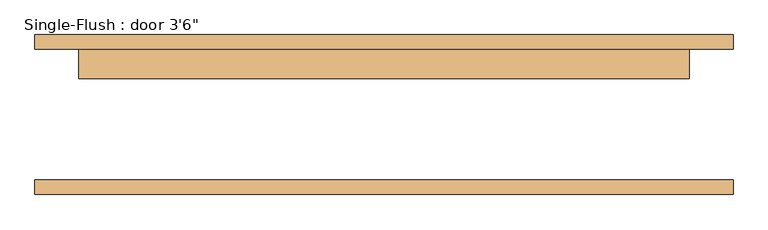
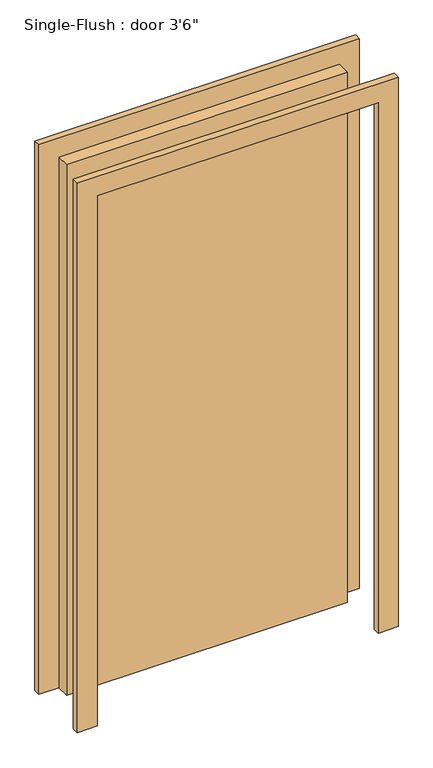
"""IFC4 building model written with IfcOpenShell, lengths in millimetres: door geometry."""

from ifc_helpers import new_model, si_unit, frame, origin, origin_with_axes, place, context, project, spatial, polyline, outline, extrude, source, transform, mapped, element, save


def door_9d399b00(model_context):
    return source(origin(), model_context, "Body", "SweptSolid", [
        extrude(outline(polyline([(2209.8, -609.6), (0.0, -609.6), (0.0, -533.4), (2133.6, -533.4), (2133.6, 533.4), (0.0, 533.4), (0.0, 609.6), (2209.8, 609.6), (2209.8, -609.6)])), frame((0.0, 114.3, 0.0), z_axis=(0.0, 1.0, 0.0), x_axis=(0.0, 0.0, 1.0)), (0.0, 0.0, 1.0), 25.4),
        extrude(outline(polyline([(2209.8, 609.6), (2209.8, -609.6), (0.0, -609.6), (0.0, -533.4), (2133.6, -533.4), (2133.6, 533.4), (0.0, 533.4), (0.0, 609.6), (2209.8, 609.6)])), frame((0.0, -139.7, 0.0), z_axis=(0.0, 1.0, 0.0), x_axis=(0.0, 0.0, 1.0)), (0.0, 0.0, 1.0), 25.4),
        extrude(outline(polyline([(533.4, 63.5), (-533.4, 63.5), (-533.4, 114.3), (533.4, 114.3), (533.4, 63.5)])), origin_with_axes(), (0.0, 0.0, 1.0), 2133.6),
    ])


if __name__ == "__main__":
    model = new_model("IFC4")
    model_context = context("Model", 3, world=origin())
    ifc_project = project(units=[si_unit("LENGTHUNIT", "METRE", prefix="MILLI")], contexts=[model_context])
    site = spatial("IfcSite", under=ifc_project)
    building = spatial("IfcBuilding", under=site)
    placement = place(None, origin())
    door_shape = door_9d399b00(model_context)
    element("IfcDoor", 1, ObjectType="Single-Flush : door 3'6\"", at=placement, inside=building, context=model_context, shape_type="MappedRepresentation", body=[
        mapped(door_shape, transform((0.0, 0.0, 0.0), x_axis=(1.0, 0.0, 0.0), y_axis=(0.0, 1.0, 0.0), z_axis=(0.0, 0.0, 1.0))),
    ])
    save(model, "model.ifc")

# Revit data of these elements
# Type "Single-Flush : door 3'6\""
#   Type Mark = "10"
#   Construction Type Id = "MDOOR"
#   Assembly Code = "C1020"
#   Analytic Construction = "Metal"
#   Thickness = 0' - 2"
#   Heat Transfer Coefficient (U) = 0.651978 BTU/(h·ft²·°F)
#   Height = 7' - 0"
#   Trim Projection Ext = 0' - 1"
#   Trim Projection Int = 0' - 1"
#   Trim Width = 0' - 3"
#   Width = 3' - 6"
#   Define Thermal Properties by = 1
#   Door Material = Door - Panel
#   Frame Material = Door - Frame
#   Visual Light Transmittance = 0
#   Solar Heat Gain Coefficient = 0
#   Function = (empty or 0)
#   Wall Closure = (empty or 0)
# Element 1 (IfcDoor, "Single-Flush : door 3'6\"")
#   Materials on its faces: "Door - Frame", "Door - Panel"
# Materials
#   "Door - Panel": class "Wood", colour RGB 210 159 95, transparency 0, Cost = 0
#   "Door - Frame": colour RGB 118 70 51, transparency 0, Cost = 0
